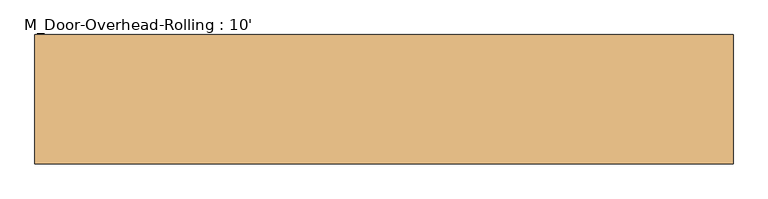
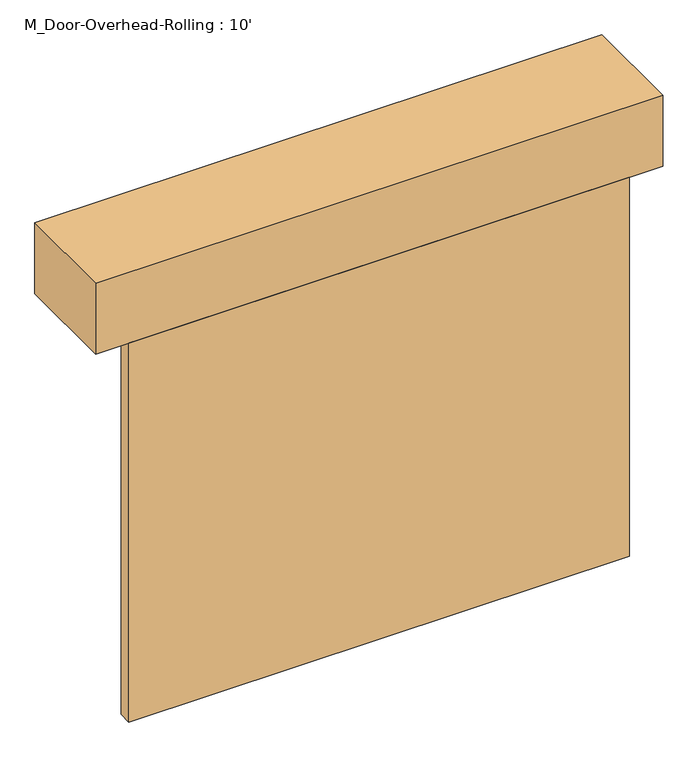
"""IFC4 building model written with IfcOpenShell, lengths in millimetres: door geometry, M_Door-Overhead-Rolling : 10'."""

from ifc_helpers import new_model, si_unit, frame, origin, origin_with_axes, place, context, project, spatial, polyline, outline, extrude, source, transform, mapped, element, save


def m_door_overhead_rolling_10_f67a646e(model_context):
    return source(origin(), model_context, "Body", "SweptSolid", [
        extrude(outline(polyline([(1524.0, 114.3), (-1524.0, 114.3), (-1524.0, 194.3), (1524.0, 194.3), (1524.0, 114.3)])), origin_with_axes(), (0.0, 0.0, 1.0), 2438.4),
        extrude(outline(polyline([(1727.2, 753.1), (1727.2, 114.3), (-1727.2, 114.3), (-1727.2, 753.1), (1727.2, 753.1)])), frame((0.0, 0.0, 2438.4), z_axis=(0.0, 0.0, 1.0), x_axis=(1.0, 0.0, 0.0)), (0.0, 0.0, 1.0), 457.2),
    ])


if __name__ == "__main__":
    model = new_model("IFC4")
    model_context = context("Model", 3, world=origin())
    ifc_project = project(units=[si_unit("LENGTHUNIT", "METRE", prefix="MILLI")], contexts=[model_context])
    site = spatial("IfcSite", under=ifc_project)
    building = spatial("IfcBuilding", under=site)
    placement = place(None, origin())
    m_door_overhead_rolling_10_shape = m_door_overhead_rolling_10_f67a646e(model_context)
    element("IfcDoor", 1, ObjectType="M_Door-Overhead-Rolling : 10'", at=placement, inside=building, context=model_context, shape_type="MappedRepresentation", body=[
        mapped(m_door_overhead_rolling_10_shape, transform((0.0, 0.0, 0.0), x_axis=(1.0, 0.0, 0.0), y_axis=(0.0, 1.0, 0.0), z_axis=(0.0, 0.0, 1.0))),
    ])
    save(model, "model.ifc")

# Revit data of these elements
# Type "M_Door-Overhead-Rolling : 10'"
#   Type Mark = "44"
#   Construction Type Id = "MDOOR"
#   Assembly Code = "B2030400"
#   Analytic Construction = "Metal"
#   Thickness = 0' - 3.14961"
#   Rough Width [instance default] = 13' - 9.35433"
#   Rough Height [instance default] = 13' - 9.35433"
#   Heat Transfer Coefficient (U) = 3.7021 W/(m²·K)
#   Height [instance default] = 13' - 9.35433"
#   Width [instance default] = 13' - 9.35433"
#   Define Thermal Properties by = 1
#   Function = 1
#   Roller Material = Steel, Paint Finish, Ivory, Matte
#   Roller Box Material = Steel, Paint Finish, Ivory, Matte
#   Visual Light Transmittance = 0
#   Solar Heat Gain Coefficient = 0
#   Wall Closure = (empty or 0)
# Element 1 (IfcDoor, "M_Door-Overhead-Rolling : 10'")
#   Rough Width = 10' - 0"
#   Rough Height = 8' - 0"
#   Height = 8' - 0"
#   Width = 10' - 0"
#   Materials on its faces: "Steel, Paint Finish, Ivory, Matte"
# Materials
#   "Steel, Paint Finish, Ivory, Matte": class "Metal", colour RGB 247 247 239, transparency 0, Description = "Steel, paint finish, ivory, matte", Cost = 0
